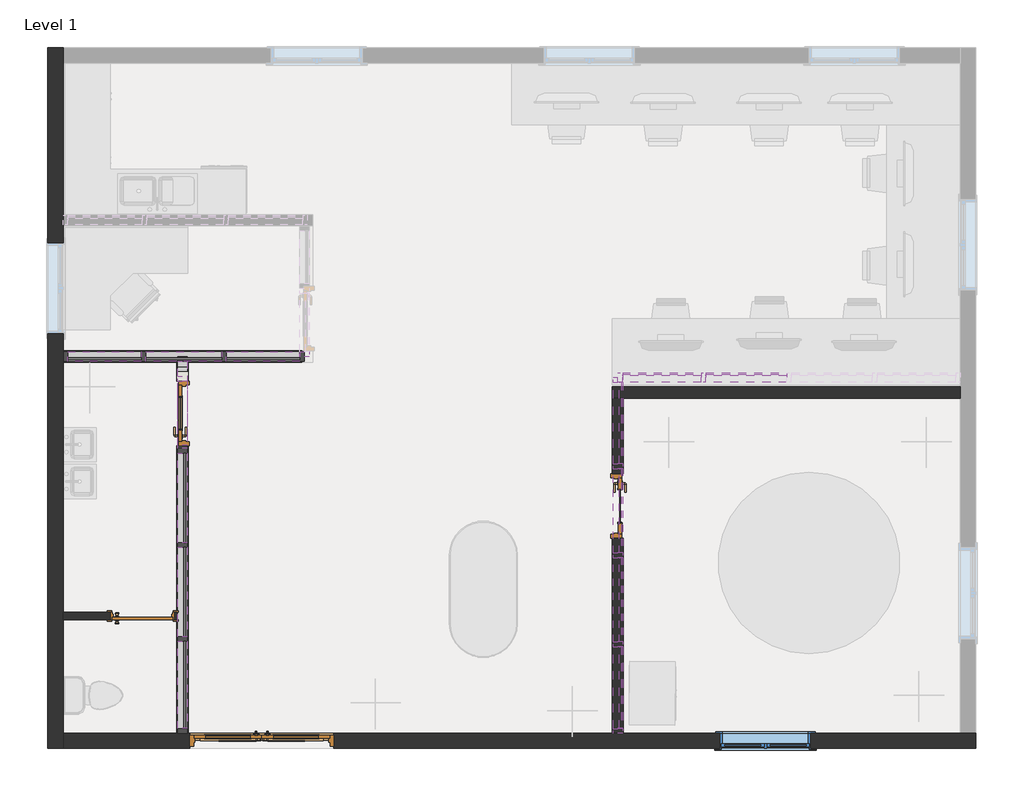
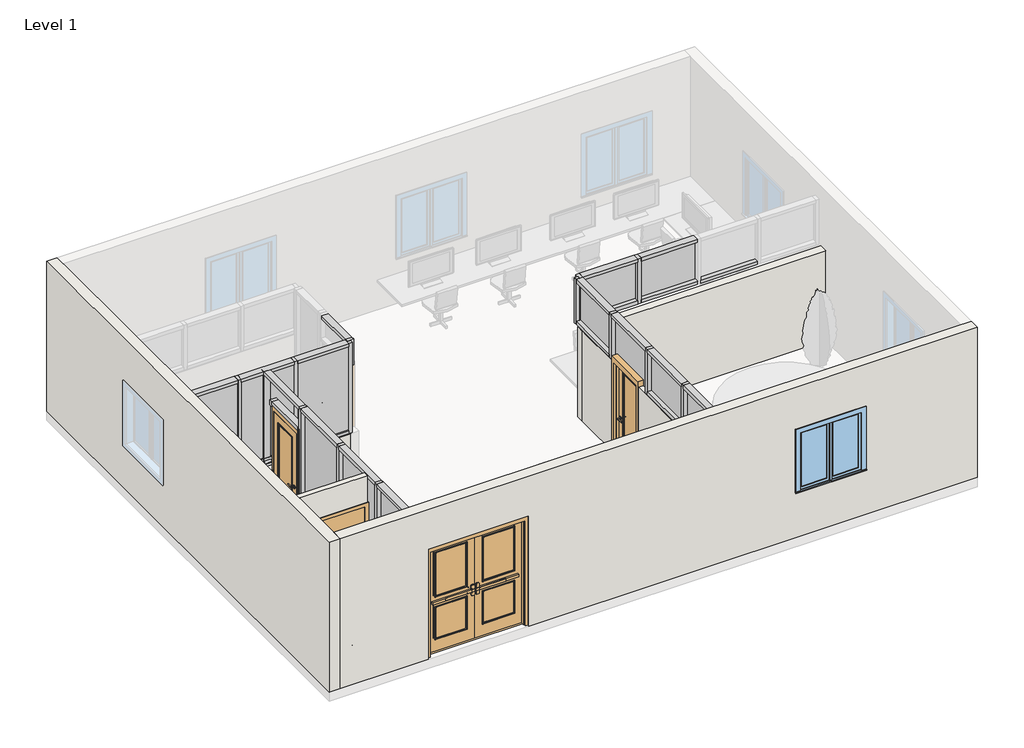
# One storey, part 1 of 2: 49 members, 12 plates, 7 walls, 4 doors, 1 window.
"""IFC4 building model written with IfcOpenShell, lengths in millimetres."""

from ifc_helpers import new_model, si_unit, frame, origin, origin_with_axes, place, context, project, spatial, polyline, outline, extrude, faceted_brep, transform, mapped, element, save
from components import door_6260e01d, door_549a8064, door_95a5efb1, door_3c591639, door_29f5c000, member_410c6227, member_73c23c35, member_7fa39cca, member_95280835, member_d60e8053, member_2fae0574, member_69c8e218, member_a08f6adc, member_3d7cb871, member_b70ee1cc, member_67d1cd44, member_476d3acb, member_e9c7f4a4, member_e1cf819f, member_429f6687, member_5446ee95, member_f5f6c3fe, member_8e09d03a, member_f1b77eba, system_panel_glazed_cfce8111, system_panel_glazed_768357cb, system_panel_glazed_3f576ca0, system_panel_glazed_47051e8e, system_panel_glazed_8590af86, system_panel_glazed_1700d241, system_panel_glazed_dd77c3d1, system_panel_glazed_5745033b, system_panel_glazed_e830b44b, window_0862ab64

model = new_model("IFC4")

# Units and contexts
model_context = context("Model", 3, world=origin())
ifc_project = project(units=[si_unit("LENGTHUNIT", "METRE", prefix="MILLI")], contexts=[model_context])

# Site, building, storey
site = spatial("IfcSite", under=ifc_project)
building = spatial("IfcBuilding", under=site)
storey = spatial("IfcBuildingStorey", under=building, Name="Level 1", Elevation=0.0)

# Doors
placement = place(None, origin())
door_shape = door_6260e01d(model_context)
door_2_shape = door_549a8064(model_context)
door_3_shape = door_95a5efb1(model_context)
element("IfcDoor", 1, ObjectType="Door-Exterior-Double-Two_Lite : 72\" x 84\"", at=placement, inside=storey, context=model_context, shape_type="MappedRepresentation", body=[
    mapped(door_shape, transform((7432.6010577, -13459.2708301, 0.0), x_axis=(1.0, 0.0, 0.0), y_axis=(0.0, 1.0, 0.0), z_axis=(0.0, 0.0, 1.0))),
    mapped(door_2_shape, transform((7432.6010577, -13459.2708301, 0.0), x_axis=(1.0, 0.0, 0.0), y_axis=(0.0, 1.0, 0.0), z_axis=(0.0, 0.0, 1.0))),
    mapped(door_3_shape, transform((7432.6010577, -13459.2708301, 0.0), x_axis=(1.0, 0.0, 0.0), y_axis=(0.0, 1.0, 0.0), z_axis=(0.0, 0.0, 1.0))),
])
door_4_shape = door_3c591639(model_context)
element("IfcDoor", 2, ObjectType="Door-Interior-Single-Flush_Panel-Wood : 32\" x 84\"", at=placement, inside=storey, context=model_context, shape_type="MappedRepresentation", body=[
    mapped(door_4_shape, transform((5832.4010577, -11779.6958301, 0.0), x_axis=(1.0, 0.0, 0.0), y_axis=(0.0, 1.0, 0.0), z_axis=(0.0, 0.0, 1.0))),
])
door_5_shape = door_29f5c000(model_context)
element("IfcDoor", 3, ObjectType="Door-Passage-Single-Full_Lite : 30\" x 84\"", at=placement, inside=storey, context=model_context, shape_type="MappedRepresentation", body=[
    mapped(door_5_shape, transform((12201.4510577, -10303.3208301, -284.48), x_axis=(0.0, -1.0, 0.0), y_axis=(1.0, 0.0, 0.0), z_axis=(0.0, 0.0, 1.0))),
])
element("IfcDoor", 4, ObjectType="Door-Passage-Single-Full_Lite : 30\" x 84\"", at=placement, inside=storey, context=model_context, shape_type="MappedRepresentation", body=[
    mapped(door_5_shape, transform((6372.1510577, -9058.7208301, 0.0), x_axis=(0.0, 1.0, 0.0), y_axis=(-1.0, 0.0, 0.0), z_axis=(0.0, 0.0, 1.0))),
])

# Members
member_shape = member_410c6227(model_context)
element("IfcMember", 5, ObjectType="Rectangular Mullion : 2.5\" x 5\" rectangular", at=placement, inside=storey, context=model_context, shape_type="MappedRepresentation", body=[
    mapped(member_shape, transform((13357.1510577, -8576.1208301, 1828.8), x_axis=(1.0, 0.0, 0.0), y_axis=(0.0, -1.0, 0.0), z_axis=(0.0, 0.0, -1.0))),
])
element("IfcMember", 6, ObjectType="Rectangular Mullion : 2.5\" x 5\" rectangular", at=placement, inside=storey, context=model_context, shape_type="MappedRepresentation", body=[
    mapped(member_shape, transform((12207.8010577, -9769.9208301, 1828.8), x_axis=(0.0, -1.0, 0.0), y_axis=(-1.0, 0.0, 0.0), z_axis=(0.0, 0.0, -1.0))),
])
element("IfcMember", 7, ObjectType="Rectangular Mullion : 2.5\" x 5\" rectangular", at=placement, inside=storey, context=model_context, shape_type="MappedRepresentation", body=[
    mapped(member_shape, transform((12207.8010577, -10963.7208301, 1828.8), x_axis=(0.0, -1.0, 0.0), y_axis=(-1.0, 0.0, 0.0), z_axis=(0.0, 0.0, -1.0))),
])
element("IfcMember", 8, ObjectType="Rectangular Mullion : 2.5\" x 5\" rectangular", at=placement, inside=storey, context=model_context, shape_type="MappedRepresentation", body=[
    mapped(member_shape, transform((12207.8010577, -12157.5208301, 1828.8), x_axis=(0.0, -1.0, 0.0), y_axis=(-1.0, 0.0, 0.0), z_axis=(0.0, 0.0, -1.0))),
])
member_2_shape = member_73c23c35(model_context)
element("IfcMember", 9, ObjectType="Rectangular Mullion : 2.5\" x 5\" rectangular", at=placement, inside=storey, context=model_context, shape_type="MappedRepresentation", body=[
    mapped(member_2_shape, transform((12207.8010577, -13351.3208301, 1828.8), x_axis=(0.0, -1.0, 0.0), y_axis=(-1.0, 0.0, 0.0), z_axis=(0.0, 0.0, -1.0))),
])
element("IfcMember", 10, ObjectType="Rectangular Mullion : 2.5\" x 5\" rectangular", at=placement, inside=storey, context=model_context, shape_type="MappedRepresentation", body=[
    mapped(member_2_shape, transform((12207.8010577, -8576.1208301, 2743.2), x_axis=(-1.0, 0.0, 0.0), y_axis=(0.0, -1.0, 0.0), z_axis=(0.0, 0.0, 1.0))),
])
element("IfcMember", 11, ObjectType="Rectangular Mullion : 2.5\" x 5\" rectangular", at=placement, inside=storey, context=model_context, shape_type="MappedRepresentation", body=[
    mapped(member_2_shape, transform((12207.8010577, -8576.1208301, 2743.2), x_axis=(0.0, 1.0, 0.0), y_axis=(-1.0, 0.0, 0.0), z_axis=(0.0, 0.0, 1.0))),
])
member_3_shape = member_7fa39cca(model_context)
element("IfcMember", 12, ObjectType="Rectangular Mullion : 2.5\" x 5\" rectangular", at=placement, inside=storey, context=model_context, shape_type="MappedRepresentation", body=[
    mapped(member_3_shape, transform((13325.4010577, -8576.1208301, 2743.2), x_axis=(0.0, 0.0, 1.0), y_axis=(0.0, -1.0, 0.0), z_axis=(1.0, 0.0, 0.0))),
])
member_4_shape = member_95280835(model_context)
element("IfcMember", 13, ObjectType="Rectangular Mullion : 2.5\" x 5\" rectangular", at=placement, inside=storey, context=model_context, shape_type="MappedRepresentation", body=[
    mapped(member_4_shape, transform((14474.7510577, -8576.1208301, 2743.2), x_axis=(0.0, 0.0, 1.0), y_axis=(0.0, -1.0, 0.0), z_axis=(1.0, 0.0, 0.0))),
])
element("IfcMember", 14, ObjectType="Rectangular Mullion : 2.5\" x 5\" rectangular", at=placement, inside=storey, context=model_context, shape_type="MappedRepresentation", body=[
    mapped(member_3_shape, transform((12271.3010577, -8576.1208301, 1828.8), x_axis=(0.0, 0.0, -1.0), y_axis=(0.0, -1.0, 0.0), z_axis=(-1.0, 0.0, 0.0))),
])
element("IfcMember", 15, ObjectType="Rectangular Mullion : 2.5\" x 5\" rectangular", at=placement, inside=storey, context=model_context, shape_type="MappedRepresentation", body=[
    mapped(member_4_shape, transform((13388.9010577, -8576.1208301, 1828.8), x_axis=(0.0, 0.0, -1.0), y_axis=(0.0, -1.0, 0.0), z_axis=(-1.0, 0.0, 0.0))),
])
element("IfcMember", 16, ObjectType="Rectangular Mullion : 2.5\" x 5\" rectangular", at=placement, inside=storey, context=model_context, shape_type="MappedRepresentation", body=[
    mapped(member_4_shape, transform((14538.2510577, -8576.1208301, 1828.8), x_axis=(0.0, 0.0, -1.0), y_axis=(0.0, -1.0, 0.0), z_axis=(-1.0, 0.0, 0.0))),
])
member_5_shape = member_d60e8053(model_context)
element("IfcMember", 17, ObjectType="Rectangular Mullion : 2.5\" x 5\" rectangular", at=placement, inside=storey, context=model_context, shape_type="MappedRepresentation", body=[
    mapped(member_5_shape, transform((6924.6010577, -8296.7208301, 914.4), x_axis=(-1.0, 0.0, 0.0), y_axis=(0.0, 1.0, 0.0), z_axis=(0.0, 0.0, -1.0))),
])
element("IfcMember", 18, ObjectType="Rectangular Mullion : 2.5\" x 5\" rectangular", at=placement, inside=storey, context=model_context, shape_type="MappedRepresentation", body=[
    mapped(member_5_shape, transform((5845.1010577, -8296.7208301, 914.4), x_axis=(-1.0, 0.0, 0.0), y_axis=(0.0, 1.0, 0.0), z_axis=(0.0, 0.0, -1.0))),
])
element("IfcMember", 19, ObjectType="Rectangular Mullion : 2.5\" x 5\" rectangular", at=placement, inside=storey, context=model_context, shape_type="MappedRepresentation", body=[
    mapped(member_5_shape, transform((6365.8010577, -9560.3708301, 914.4), x_axis=(0.0, -1.0, 0.0), y_axis=(-1.0, 0.0, 0.0), z_axis=(0.0, 0.0, -1.0))),
])
element("IfcMember", 20, ObjectType="Rectangular Mullion : 2.5\" x 5\" rectangular", at=placement, inside=storey, context=model_context, shape_type="MappedRepresentation", body=[
    mapped(member_5_shape, transform((6365.8010577, -10824.0208301, 914.4), x_axis=(0.0, -1.0, 0.0), y_axis=(-1.0, 0.0, 0.0), z_axis=(0.0, 0.0, -1.0))),
])
element("IfcMember", 21, ObjectType="Rectangular Mullion : 2.5\" x 5\" rectangular", at=placement, inside=storey, context=model_context, shape_type="MappedRepresentation", body=[
    mapped(member_5_shape, transform((6365.8010577, -12087.6708301, 914.4), x_axis=(0.0, -1.0, 0.0), y_axis=(-1.0, 0.0, 0.0), z_axis=(0.0, 0.0, -1.0))),
])
member_6_shape = member_2fae0574(model_context)
element("IfcMember", 22, ObjectType="Rectangular Mullion : 2.5\" x 5\" rectangular", at=placement, inside=storey, context=model_context, shape_type="MappedRepresentation", body=[
    mapped(member_6_shape, transform((4765.6010577, -8296.7208301, 914.4), x_axis=(-1.0, 0.0, 0.0), y_axis=(0.0, 1.0, 0.0), z_axis=(0.0, 0.0, -1.0))),
])
element("IfcMember", 23, ObjectType="Rectangular Mullion : 2.5\" x 5\" rectangular", at=placement, inside=storey, context=model_context, shape_type="MappedRepresentation", body=[
    mapped(member_6_shape, transform((6365.8010577, -13351.3208301, 914.4), x_axis=(0.0, -1.0, 0.0), y_axis=(-1.0, 0.0, 0.0), z_axis=(0.0, 0.0, -1.0))),
])
element("IfcMember", 24, ObjectType="Rectangular Mullion : 2.5\" x 5\" rectangular", at=placement, inside=storey, context=model_context, shape_type="MappedRepresentation", body=[
    mapped(member_6_shape, transform((8004.1010577, -8296.7208301, 2743.2), x_axis=(1.0, 0.0, 0.0), y_axis=(0.0, 1.0, 0.0), z_axis=(0.0, 0.0, 1.0))),
])
member_7_shape = member_69c8e218(model_context)
element("IfcMember", 25, ObjectType="Rectangular Mullion : 2.5\" x 5\" rectangular", at=placement, inside=storey, context=model_context, shape_type="MappedRepresentation", body=[
    mapped(member_7_shape, transform((12207.8010577, -13287.8208301, 2743.2), x_axis=(0.0, 0.0, 1.0), y_axis=(-1.0, 0.0, 0.0), z_axis=(0.0, -1.0, 0.0))),
])
element("IfcMember", 26, ObjectType="Rectangular Mullion : 2.5\" x 5\" rectangular", at=placement, inside=storey, context=model_context, shape_type="MappedRepresentation", body=[
    mapped(member_7_shape, transform((12207.8010577, -9738.1708301, 2743.2), x_axis=(0.0, 0.0, 1.0), y_axis=(-1.0, 0.0, 0.0), z_axis=(0.0, -1.0, 0.0))),
])
member_8_shape = member_a08f6adc(model_context)
element("IfcMember", 27, ObjectType="Rectangular Mullion : 2.5\" x 5\" rectangular", at=placement, inside=storey, context=model_context, shape_type="MappedRepresentation", body=[
    mapped(member_8_shape, transform((12207.8010577, -10931.9708301, 2743.2), x_axis=(0.0, 0.0, 1.0), y_axis=(-1.0, 0.0, 0.0), z_axis=(0.0, -1.0, 0.0))),
])
element("IfcMember", 28, ObjectType="Rectangular Mullion : 2.5\" x 5\" rectangular", at=placement, inside=storey, context=model_context, shape_type="MappedRepresentation", body=[
    mapped(member_8_shape, transform((12207.8010577, -12125.7708301, 2743.2), x_axis=(0.0, 0.0, 1.0), y_axis=(-1.0, 0.0, 0.0), z_axis=(0.0, -1.0, 0.0))),
])
element("IfcMember", 29, ObjectType="Rectangular Mullion : 2.5\" x 5\" rectangular", at=placement, inside=storey, context=model_context, shape_type="MappedRepresentation", body=[
    mapped(member_7_shape, transform((12207.8010577, -8639.6208301, 1828.8), x_axis=(0.0, 0.0, -1.0), y_axis=(-1.0, 0.0, 0.0), z_axis=(0.0, 1.0, 0.0))),
])
element("IfcMember", 30, ObjectType="Rectangular Mullion : 2.5\" x 5\" rectangular", at=placement, inside=storey, context=model_context, shape_type="MappedRepresentation", body=[
    mapped(member_7_shape, transform((12207.8010577, -12189.2708301, 1828.8), x_axis=(0.0, 0.0, -1.0), y_axis=(-1.0, 0.0, 0.0), z_axis=(0.0, 1.0, 0.0))),
])
element("IfcMember", 31, ObjectType="Rectangular Mullion : 2.5\" x 5\" rectangular", at=placement, inside=storey, context=model_context, shape_type="MappedRepresentation", body=[
    mapped(member_8_shape, transform((12207.8010577, -10995.4708301, 1828.8), x_axis=(0.0, 0.0, -1.0), y_axis=(-1.0, 0.0, 0.0), z_axis=(0.0, 1.0, 0.0))),
])
member_9_shape = member_3d7cb871(model_context)
element("IfcMember", 32, ObjectType="Rectangular Mullion : 2.5\" x 5\" rectangular", at=placement, inside=storey, context=model_context, shape_type="MappedRepresentation", body=[
    mapped(member_9_shape, transform((6365.8010577, -8360.2208301, 863.6), x_axis=(0.0, 0.0, -1.0), y_axis=(-1.0, 0.0, 0.0), z_axis=(0.0, 1.0, 0.0))),
])
member_10_shape = member_b70ee1cc(model_context)
element("IfcMember", 33, ObjectType="Rectangular Mullion : 2.5\" x 5\" rectangular", at=placement, inside=storey, context=model_context, shape_type="MappedRepresentation", body=[
    mapped(member_10_shape, transform((6365.8010577, -8626.9208301, 2235.2), x_axis=(0.0, 0.0, -1.0), y_axis=(-1.0, 0.0, 0.0), z_axis=(0.0, 1.0, 0.0))),
])
element("IfcMember", 34, ObjectType="Rectangular Mullion : 2.5\" x 5\" rectangular", at=placement, inside=storey, context=model_context, shape_type="MappedRepresentation", body=[
    mapped(member_6_shape, transform((6365.8010577, -8296.7208301, 2743.2), x_axis=(0.0, 1.0, 0.0), y_axis=(-1.0, 0.0, 0.0), z_axis=(0.0, 0.0, 1.0))),
])
member_11_shape = member_67d1cd44(model_context)
element("IfcMember", 35, ObjectType="Rectangular Mullion : 2.5\" x 5\" rectangular", at=placement, inside=storey, context=model_context, shape_type="MappedRepresentation", body=[
    mapped(member_11_shape, transform((6365.8010577, -8296.7208301, 914.4), x_axis=(0.0, 1.0, 0.0), y_axis=(-1.0, 0.0, 0.0), z_axis=(0.0, 0.0, 1.0))),
])
member_12_shape = member_476d3acb(model_context)
element("IfcMember", 36, ObjectType="Rectangular Mullion : 2.5\" x 5\" rectangular", at=placement, inside=storey, context=model_context, shape_type="MappedRepresentation", body=[
    mapped(member_12_shape, transform((6365.8010577, -13287.8208301, 2743.2), x_axis=(0.0, 0.0, 1.0), y_axis=(-1.0, 0.0, 0.0), z_axis=(0.0, -1.0, 0.0))),
])
element("IfcMember", 37, ObjectType="Rectangular Mullion : 2.5\" x 5\" rectangular", at=placement, inside=storey, context=model_context, shape_type="MappedRepresentation", body=[
    mapped(member_12_shape, transform((6365.8010577, -9528.6208301, 2743.2), x_axis=(0.0, 0.0, 1.0), y_axis=(-1.0, 0.0, 0.0), z_axis=(0.0, -1.0, 0.0))),
])
member_13_shape = member_e9c7f4a4(model_context)
element("IfcMember", 38, ObjectType="Rectangular Mullion : 2.5\" x 5\" rectangular", at=placement, inside=storey, context=model_context, shape_type="MappedRepresentation", body=[
    mapped(member_13_shape, transform((6365.8010577, -10792.2708301, 2743.2), x_axis=(0.0, 0.0, 1.0), y_axis=(-1.0, 0.0, 0.0), z_axis=(0.0, -1.0, 0.0))),
])
element("IfcMember", 39, ObjectType="Rectangular Mullion : 2.5\" x 5\" rectangular", at=placement, inside=storey, context=model_context, shape_type="MappedRepresentation", body=[
    mapped(member_13_shape, transform((6365.8010577, -12055.9208301, 2743.2), x_axis=(0.0, 0.0, 1.0), y_axis=(-1.0, 0.0, 0.0), z_axis=(0.0, -1.0, 0.0))),
])
element("IfcMember", 40, ObjectType="Rectangular Mullion : 2.5\" x 5\" rectangular", at=placement, inside=storey, context=model_context, shape_type="MappedRepresentation", body=[
    mapped(member_13_shape, transform((6365.8010577, -9592.1208301, 914.4), x_axis=(0.0, 0.0, -1.0), y_axis=(-1.0, 0.0, 0.0), z_axis=(0.0, 1.0, 0.0))),
])
element("IfcMember", 41, ObjectType="Rectangular Mullion : 2.5\" x 5\" rectangular", at=placement, inside=storey, context=model_context, shape_type="MappedRepresentation", body=[
    mapped(member_13_shape, transform((6365.8010577, -10855.7708301, 914.4), x_axis=(0.0, 0.0, -1.0), y_axis=(-1.0, 0.0, 0.0), z_axis=(0.0, 1.0, 0.0))),
])
element("IfcMember", 42, ObjectType="Rectangular Mullion : 2.5\" x 5\" rectangular", at=placement, inside=storey, context=model_context, shape_type="MappedRepresentation", body=[
    mapped(member_12_shape, transform((6365.8010577, -12119.4208301, 914.4), x_axis=(0.0, 0.0, -1.0), y_axis=(-1.0, 0.0, 0.0), z_axis=(0.0, 1.0, 0.0))),
])
member_14_shape = member_e1cf819f(model_context)
element("IfcMember", 43, ObjectType="Rectangular Mullion : 2.5\" x 5\" rectangular", at=placement, inside=storey, context=model_context, shape_type="MappedRepresentation", body=[
    mapped(member_14_shape, transform((6365.8010577, -9490.5208301, 2298.7), x_axis=(0.0, 1.0, 0.0), y_axis=(-1.0, 0.0, 0.0), z_axis=(0.0, 0.0, 1.0))),
])
member_15_shape = member_429f6687(model_context)
element("IfcMember", 44, ObjectType="Rectangular Mullion : 2.5\" x 5\" rectangular", at=placement, inside=storey, context=model_context, shape_type="MappedRepresentation", body=[
    mapped(member_15_shape, transform((8004.1010577, -8233.2208301, 2754.1090709), x_axis=(0.0, 0.0, 1.0), y_axis=(-1.0, 0.0, 0.0), z_axis=(0.0, -1.0, 0.0))),
])
element("IfcMember", 45, ObjectType="Rectangular Mullion : 2.5\" x 5\" rectangular", at=placement, inside=storey, context=model_context, shape_type="MappedRepresentation", body=[
    mapped(member_11_shape, transform((6365.8010577, -8499.9208301, 863.6), x_axis=(0.0, -1.0, 0.0), y_axis=(-1.0, 0.0, 0.0), z_axis=(0.0, 0.0, -1.0))),
])
member_16_shape = member_5446ee95(model_context)
element("IfcMember", 46, ObjectType="Rectangular Mullion : 2.5\" x 5\" rectangular", at=placement, inside=storey, context=model_context, shape_type="MappedRepresentation", body=[
    mapped(member_16_shape, transform((6365.8010577, -8626.9208301, 2197.7952723), x_axis=(0.0, -1.0, 0.0), y_axis=(-1.0, 0.0, 0.0), z_axis=(0.0, 0.0, -1.0))),
])
member_17_shape = member_f5f6c3fe(model_context)
element("IfcMember", 47, ObjectType="Rectangular Mullion : 2.5\" x 5\" rectangular", at=placement, inside=storey, context=model_context, shape_type="MappedRepresentation", body=[
    mapped(member_17_shape, transform((4829.1010577, -8296.7208301, 2743.2), x_axis=(0.0, 0.0, 1.0), y_axis=(0.0, 1.0, 0.0), z_axis=(-1.0, 0.0, 0.0))),
])
element("IfcMember", 48, ObjectType="Rectangular Mullion : 2.5\" x 5\" rectangular", at=placement, inside=storey, context=model_context, shape_type="MappedRepresentation", body=[
    mapped(member_17_shape, transform((6956.3510577, -8296.7208301, 2743.2), x_axis=(0.0, 0.0, 1.0), y_axis=(0.0, 1.0, 0.0), z_axis=(-1.0, 0.0, 0.0))),
])
member_18_shape = member_8e09d03a(model_context)
element("IfcMember", 49, ObjectType="Rectangular Mullion : 2.5\" x 5\" rectangular", at=placement, inside=storey, context=model_context, shape_type="MappedRepresentation", body=[
    mapped(member_18_shape, transform((5876.8510577, -8296.7208301, 2743.2), x_axis=(0.0, 0.0, 1.0), y_axis=(0.0, 1.0, 0.0), z_axis=(-1.0, 0.0, 0.0))),
])
element("IfcMember", 50, ObjectType="Rectangular Mullion : 2.5\" x 5\" rectangular", at=placement, inside=storey, context=model_context, shape_type="MappedRepresentation", body=[
    mapped(member_17_shape, transform((7940.6010577, -8296.7208301, 914.4), x_axis=(0.0, 0.0, -1.0), y_axis=(0.0, 1.0, 0.0), z_axis=(1.0, 0.0, 0.0))),
])
element("IfcMember", 51, ObjectType="Rectangular Mullion : 2.5\" x 5\" rectangular", at=placement, inside=storey, context=model_context, shape_type="MappedRepresentation", body=[
    mapped(member_17_shape, transform((5813.3510577, -8296.7208301, 914.4), x_axis=(0.0, 0.0, -1.0), y_axis=(0.0, 1.0, 0.0), z_axis=(1.0, 0.0, 0.0))),
])
element("IfcMember", 52, ObjectType="Rectangular Mullion : 2.5\" x 5\" rectangular", at=placement, inside=storey, context=model_context, shape_type="MappedRepresentation", body=[
    mapped(member_18_shape, transform((6892.8510577, -8296.7208301, 914.4), x_axis=(0.0, 0.0, -1.0), y_axis=(0.0, 1.0, 0.0), z_axis=(1.0, 0.0, 0.0))),
])
member_19_shape = member_f1b77eba(model_context)
element("IfcMember", 53, ObjectType="Rectangular Mullion : 2.5\" x 5\" rectangular", at=placement, inside=storey, context=model_context, shape_type="MappedRepresentation", body=[
    mapped(member_19_shape, transform((8004.1010577, -8296.7208301, 2235.2), x_axis=(0.0, -1.0, 0.0), y_axis=(-1.0, 0.0, 0.0), z_axis=(0.0, 0.0, -1.0))),
])

# Plates
system_panel_glazed_shape = system_panel_glazed_cfce8111(model_context)
element("IfcPlate", 54, ObjectType="System Panel : Glazed", at=placement, inside=storey, context=model_context, shape_type="MappedRepresentation", body=[
    mapped(system_panel_glazed_shape, transform((12798.3510577, -8576.1208301, 1892.3), x_axis=(1.0, 0.0, 0.0), y_axis=(0.0, 1.0, 0.0), z_axis=(0.0, 0.0, 1.0))),
])
system_panel_glazed_2_shape = system_panel_glazed_768357cb(model_context)
element("IfcPlate", 55, ObjectType="System Panel : Glazed", at=placement, inside=storey, context=model_context, shape_type="MappedRepresentation", body=[
    mapped(system_panel_glazed_2_shape, transform((13931.8260577, -8576.1208301, 1892.3), x_axis=(1.0, 0.0, 0.0), y_axis=(0.0, 1.0, 0.0), z_axis=(0.0, 0.0, 1.0))),
])
system_panel_glazed_3_shape = system_panel_glazed_3f576ca0(model_context)
element("IfcPlate", 56, ObjectType="System Panel : Glazed", at=placement, inside=storey, context=model_context, shape_type="MappedRepresentation", body=[
    mapped(system_panel_glazed_3_shape, transform((12207.8010577, -9188.8958301, 1892.3), x_axis=(0.0, -1.0, 0.0), y_axis=(1.0, 0.0, 0.0), z_axis=(0.0, 0.0, 1.0))),
])
element("IfcPlate", 57, ObjectType="System Panel : Glazed", at=placement, inside=storey, context=model_context, shape_type="MappedRepresentation", body=[
    mapped(system_panel_glazed_3_shape, transform((12207.8010577, -12738.5458301, 1892.3), x_axis=(0.0, -1.0, 0.0), y_axis=(1.0, 0.0, 0.0), z_axis=(0.0, 0.0, 1.0))),
])
system_panel_glazed_4_shape = system_panel_glazed_47051e8e(model_context)
element("IfcPlate", 58, ObjectType="System Panel : Glazed", at=placement, inside=storey, context=model_context, shape_type="MappedRepresentation", body=[
    mapped(system_panel_glazed_4_shape, transform((12207.8010577, -11560.6208301, 1892.3), x_axis=(0.0, -1.0, 0.0), y_axis=(1.0, 0.0, 0.0), z_axis=(0.0, 0.0, 1.0))),
])
system_panel_glazed_5_shape = system_panel_glazed_8590af86(model_context)
element("IfcPlate", 59, ObjectType="System Panel : Glazed", at=placement, inside=storey, context=model_context, shape_type="MappedRepresentation", body=[
    mapped(system_panel_glazed_5_shape, transform((6365.8010577, -10192.1958301, 977.9), x_axis=(0.0, -1.0, 0.0), y_axis=(1.0, 0.0, 0.0), z_axis=(0.0, 0.0, 1.0))),
])
element("IfcPlate", 60, ObjectType="System Panel : Glazed", at=placement, inside=storey, context=model_context, shape_type="MappedRepresentation", body=[
    mapped(system_panel_glazed_5_shape, transform((6365.8010577, -11455.8458301, 977.9), x_axis=(0.0, -1.0, 0.0), y_axis=(1.0, 0.0, 0.0), z_axis=(0.0, 0.0, 1.0))),
])
system_panel_glazed_6_shape = system_panel_glazed_1700d241(model_context)
element("IfcPlate", 61, ObjectType="System Panel : Glazed", at=placement, inside=storey, context=model_context, shape_type="MappedRepresentation", body=[
    mapped(system_panel_glazed_6_shape, transform((6365.8010577, -12703.6208301, 977.9), x_axis=(0.0, -1.0, 0.0), y_axis=(1.0, 0.0, 0.0), z_axis=(0.0, 0.0, 1.0))),
])
system_panel_glazed_7_shape = system_panel_glazed_dd77c3d1(model_context)
element("IfcPlate", 62, ObjectType="System Panel : Glazed", at=placement, inside=storey, context=model_context, shape_type="MappedRepresentation", body=[
    mapped(system_panel_glazed_7_shape, transform((12207.8010577, -10366.8208301, 1828.8), x_axis=(0.0, -1.0, 0.0), y_axis=(1.0, 0.0, 0.0), z_axis=(0.0, 0.0, 1.0))),
])
system_panel_glazed_8_shape = system_panel_glazed_5745033b(model_context)
element("IfcPlate", 63, ObjectType="System Panel : Glazed", at=placement, inside=storey, context=model_context, shape_type="MappedRepresentation", body=[
    mapped(system_panel_glazed_8_shape, transform((7448.4760577, -8296.7208301, 977.9), x_axis=(-1.0, 0.0, 0.0), y_axis=(0.0, -1.0, 0.0), z_axis=(0.0, 0.0, 1.0))),
])
element("IfcPlate", 64, ObjectType="System Panel : Glazed", at=placement, inside=storey, context=model_context, shape_type="MappedRepresentation", body=[
    mapped(system_panel_glazed_8_shape, transform((5321.2260577, -8296.7208301, 977.9), x_axis=(-1.0, 0.0, 0.0), y_axis=(0.0, -1.0, 0.0), z_axis=(0.0, 0.0, 1.0))),
])
system_panel_glazed_9_shape = system_panel_glazed_e830b44b(model_context)
element("IfcPlate", 65, ObjectType="System Panel : Glazed", at=placement, inside=storey, context=model_context, shape_type="MappedRepresentation", body=[
    mapped(system_panel_glazed_9_shape, transform((6384.8510577, -8296.7208301, 977.9), x_axis=(-1.0, 0.0, 0.0), y_axis=(0.0, -1.0, 0.0), z_axis=(0.0, 0.0, 1.0))),
])

# Walls
element("IfcWall", 66, ObjectType="Generic - 4\" Brick", at=placement, inside=storey, context=model_context, shape_type="SweptSolid", body=[
    extrude(outline(polyline([(2743.2, 6289.6010577), (2743.2, 4765.6010577), (0.0, 4765.6010577), (0.0, 5400.6010577), (2159.0, 5400.6010577), (2159.0, 6264.2010577), (0.0, 6264.2010577), (0.0, 6289.6010577), (2743.2, 6289.6010577)])), frame((0.0, -11827.3208301, 0.0), z_axis=(0.0, 1.0, 0.0), x_axis=(0.0, 0.0, 1.0)), (0.0, 0.0, 1.0), 101.6),
])
element("IfcWall", 67, ObjectType="Generic - 6\"", at=placement, inside=storey, context=model_context, shape_type="Brep", body=[
    faceted_brep([(7966.0010577, -8220.5208301, 0.0), (4765.6010577, -8220.5208301, 0.0), (4765.6010577, -8220.5208301, 914.4), (7966.0010577, -8220.5208301, 914.4), (7966.0010577, -8372.9208301, 0.0), (7966.0010577, -8372.9208301, 914.4), (6442.0010577, -8372.9208301, 914.4), (6289.6010577, -8372.9208301, 914.4), (4765.6010577, -8372.9208301, 914.4), (4765.6010577, -8372.9208301, 0.0), (6289.6010577, -8372.9208301, 0.0), (6442.0010577, -8372.9208301, 0.0)], [[[0, 1, 2, 3]], [[4, 5, 6, 7, 8, 9, 10, 11]], [[1, 0, 4, 11, 10, 9]], [[3, 2, 8, 7, 6, 5]], [[0, 3, 5, 4]], [[2, 1, 9, 8]]]),
])
element("IfcWall", 68, ObjectType="Generic - 6\"", at=placement, inside=storey, context=model_context, shape_type="Brep", body=[
    faceted_brep([(6289.6010577, -13351.3208301, 0.0), (6289.6010577, -13351.3208301, 914.4), (6289.6010577, -9490.5208301, 914.4), (6289.6010577, -9490.5208301, 0.0), (6289.6010577, -11725.7208301, 0.0), (6289.6010577, -11827.3208301, 0.0), (6442.0010577, -13351.3208301, 914.4), (6442.0010577, -13351.3208301, 0.0), (6442.0010577, -9490.5208301, 0.0), (6442.0010577, -9490.5208301, 914.4)], [[[0, 1, 2, 3, 4, 5]], [[6, 7, 8, 9]], [[7, 0, 5, 4, 3, 8]], [[1, 6, 9, 2]], [[1, 0, 7, 6]], [[3, 2, 9, 8]]]),
    faceted_brep([(6289.6010577, -8372.9208301, 0.0), (6289.6010577, -8626.9208301, 0.0), (6289.6010577, -8626.9208301, 914.4), (6289.6010577, -8499.9208301, 914.4), (6289.6010577, -8499.9208301, 863.6), (6289.6010577, -8372.9208301, 863.6), (6442.0010577, -8626.9208301, 0.0), (6442.0010577, -8372.9208301, 0.0), (6442.0010577, -8372.9208301, 863.6), (6442.0010577, -8499.9208301, 863.6), (6442.0010577, -8499.9208301, 914.4), (6442.0010577, -8626.9208301, 914.4)], [[[0, 1, 2, 3, 4, 5]], [[6, 7, 8, 9, 10, 11]], [[0, 7, 6, 1]], [[2, 11, 10, 3]], [[7, 0, 5, 8]], [[2, 1, 6, 11]], [[9, 4, 3, 10]], [[4, 9, 8, 5]]]),
])
element("IfcWall", 69, ObjectType="Generic - 6\"", at=placement, inside=storey, context=model_context, shape_type="Brep", body=[
    faceted_brep([(16805.2010577, -8703.1208301, 0.0), (12131.6010577, -8703.1208301, 0.0), (12131.6010577, -8703.1208301, 1828.8), (16805.2010577, -8703.1208301, 1828.8), (16805.2010577, -8855.5208301, 0.0), (16805.2010577, -8855.5208301, 1828.8), (12284.0010577, -8855.5208301, 1828.8), (12131.6010577, -8855.5208301, 1828.8), (12131.6010577, -8855.5208301, 0.0), (12284.0010577, -8855.5208301, 0.0)], [[[0, 1, 2, 3]], [[4, 5, 6, 7, 8, 9]], [[1, 0, 4, 9, 8]], [[3, 2, 7, 6, 5]], [[0, 3, 5, 4]], [[2, 1, 8, 7]]]),
])
element("IfcWall", 70, ObjectType="Generic - 6\"", at=placement, inside=storey, context=model_context, shape_type="SweptSolid", body=[
    extrude(outline(polyline([(12284.0010577, -13351.3208301), (12131.6010577, -13351.3208301), (12131.6010577, -10735.1208301), (12284.0010577, -10735.1208301), (12284.0010577, -13351.3208301)])), origin_with_axes(), (0.0, 0.0, 1.0), 1828.8),
    extrude(outline(polyline([(12131.6010577, -8855.5208301), (12284.0010577, -8855.5208301), (12284.0010577, -9871.5208301), (12131.6010577, -9871.5208301), (12131.6010577, -8855.5208301)])), origin_with_axes(), (0.0, 0.0, 1.0), 1828.8),
])
element("IfcWall", 71, ObjectType="Generic - 8\"", at=placement, inside=storey, context=model_context, shape_type="Brep", body=[
    faceted_brep([(4562.4010577, -4156.5208301, 0.0), (4562.4010577, -13554.5208301, 0.0), (4562.4010577, -13554.5208301, 3048.0), (4562.4010577, -4156.5208301, 3048.0), (4562.4010577, -7991.9208301, 2133.6), (4562.4010577, -7991.9208301, 914.4), (4562.4010577, -6772.7208301, 914.4), (4562.4010577, -6772.7208301, 2133.6), (4765.6010577, -4156.5208301, 0.0), (4765.6010577, -4156.5208301, 3048.0), (4765.6010577, -4359.7208301, 3048.0), (4765.6010577, -13351.3208301, 3048.0), (4765.6010577, -13554.5208301, 3048.0), (4765.6010577, -13554.5208301, 0.0), (4765.6010577, -13351.3208301, 0.0), (4765.6010577, -11827.3208301, 0.0), (4765.6010577, -11725.7208301, 0.0), (4765.6010577, -8372.9208301, 0.0), (4765.6010577, -8220.5208301, 0.0), (4765.6010577, -6544.1208301, 0.0), (4765.6010577, -6391.7208301, 0.0), (4765.6010577, -4359.7208301, 0.0), (4765.6010577, -7991.9208301, 2133.6), (4765.6010577, -6772.7208301, 2133.6), (4765.6010577, -6772.7208301, 914.4), (4765.6010577, -7991.9208301, 914.4)], [[[0, 1, 2, 3], [4, 5, 6, 7]], [[8, 9, 10, 11, 12, 13, 14, 15, 16, 17, 18, 19, 20, 21], [22, 23, 24, 25]], [[1, 0, 8, 21, 20, 19, 18, 17, 16, 15, 14, 13]], [[3, 2, 12, 11, 10, 9]], [[2, 1, 13, 12]], [[0, 3, 9, 8]], [[5, 4, 22, 25]], [[6, 5, 25, 24]], [[7, 6, 24, 23]], [[4, 7, 23, 22]]]),
])
element("IfcWall", 72, ObjectType="Generic - 8\"", at=placement, inside=storey, context=model_context, shape_type="Brep", body=[
    faceted_brep([(17008.4010577, -13554.5208301, 3048.0), (4765.6010577, -13554.5208301, 3048.0), (4765.6010577, -13554.5208301, 0.0), (6467.4010577, -13554.5208301, 0.0), (6467.4010577, -13554.5208301, 2235.2), (8397.8010577, -13554.5208301, 2235.2), (8397.8010577, -13554.5208301, 0.0), (17008.4010577, -13554.5208301, 0.0), (13579.4010577, -13554.5208301, 2133.6), (14798.6010577, -13554.5208301, 2133.6), (14798.6010577, -13554.5208301, 914.4), (13579.4010577, -13554.5208301, 914.4), (4765.6010577, -13351.3208301, 3048.0), (16805.2010577, -13351.3208301, 3048.0), (17008.4010577, -13351.3208301, 3048.0), (17008.4010577, -13351.3208301, 0.0), (16805.2010577, -13351.3208301, 0.0), (12284.0010577, -13351.3208301, 0.0), (12131.6010577, -13351.3208301, 0.0), (8397.8010577, -13351.3208301, 0.0), (8397.8010577, -13351.3208301, 2235.2), (6467.4010577, -13351.3208301, 2235.2), (6467.4010577, -13351.3208301, 0.0), (6442.0010577, -13351.3208301, 0.0), (6289.6010577, -13351.3208301, 0.0), (4765.6010577, -13351.3208301, 0.0), (13579.4010577, -13351.3208301, 2133.6), (13579.4010577, -13351.3208301, 914.4), (14798.6010577, -13351.3208301, 914.4), (14798.6010577, -13351.3208301, 2133.6)], [[[0, 1, 2, 3, 4, 5, 6, 7], [8, 9, 10, 11]], [[12, 13, 14, 15, 16, 17, 18, 19, 20, 21, 22, 23, 24, 25], [26, 27, 28, 29]], [[2, 25, 24, 23, 22, 3]], [[15, 7, 6, 19, 18, 17, 16]], [[1, 0, 14, 13, 12]], [[2, 1, 12, 25]], [[0, 7, 15, 14]], [[5, 20, 19, 6]], [[20, 5, 4, 21]], [[21, 4, 3, 22]], [[27, 26, 8, 11]], [[28, 27, 11, 10]], [[29, 28, 10, 9]], [[26, 29, 9, 8]]]),
])

# Window
window_shape = window_0862ab64(model_context)
element("IfcWindow", 73, ObjectType="Casement Dbl with Trim : 48\" x 48\"", at=placement, inside=storey, context=model_context, shape_type="MappedRepresentation", body=[
    mapped(window_shape, transform((14189.0010577, -13433.8708301, 0.0), x_axis=(-1.0, 0.0, 0.0), y_axis=(0.0, -1.0, 0.0), z_axis=(0.0, 0.0, 1.0))),
])

save(model, "model.ifc")

# Revit data of these elements
# Type "Door-Exterior-Double-Two_Lite : 72\" x 84\""
#   Type Mark = "8"
#   Assembly Code = "B2030100"
#   Analytic Construction = "Metal frame, double glass door"
#   Top Rail = 0' - 4 5/8"
#   Threshold Length [instance default] = 6' - 4"
#   Threshold Offset [instance default] = 0' - 0 1/2"
#   Thickness = 0' - 1 3/4"
#   Thermal Resistance (R) = 1.3794 (h·ft²·°F)/BTU
#   Swing Angle [instance default] = 90.00°
#   Strike Height = 3' - 4"
#   Stiles = 0' - 6"
#   SinglePanelWidth = 3' - 0"
#   Rough Width [instance default] = 6' - 4"
#   Rough Height [instance default] = 7' - 4"
#   MFOpeningHeight [instance default] = 0' - 4"
#   MFOpeningWidth [instance default] = 0' - 4"
#   Lock Rail = 0' - 8"
#   Inset Calculate [instance default] = 0' - 4"
#   Masonry Inset [instance default] = 0' - 1"
#   Height = 7' - 0"
#   Width = 6' - 0"
#   Heat Transfer Coefficient (U) = 0.7250 BTU/(h·ft²·°F)
#   Glass Thickness = 0' - 0 3/4"
#   Masonry Frame Depth = 0' - 5 3/4"
#   Bottom Rail = 0' - 10"
#   Threshold [instance default] = yes
#   Masonry Frame [instance default] = yes
#   Function = 1
#   Dry Wall Frame [instance default] = no
#   Threshold Material = none
#   Panic Bar Material = Metal - Stainless Steel
#   Panel Material = Metal - Painted - Grey
#   Glass Stop Material = Metal - Painted - Grey
#   Frame Material = Metal - Painted - Grey
#   Exterior Pull Material = Metal - Stainless Steel
#   Visual Light Transmittance = 0
#   Solar Heat Gain Coefficient = 0
#   Wall Closure = (empty or 0)
# Type "Door-Interior-Single-Flush_Panel-Wood : 32\" x 84\""
#   Type Mark = "11"
#   Assembly Code = "C1020300"
#   Analytic Construction = "Wooden"
#   Thickness = 0' - 1 3/8"
#   Thermal Resistance (R) = 2.5876 (h·ft²·°F)/BTU
#   Swing Angle [instance default] = 90.00°
#   Rough Width = 2' - 10"
#   Rough Height = 7' - 1"
#   Height = 7' - 0"
#   Width = 2' - 8"
#   Heat Transfer Coefficient (U) = 0.3865 BTU/(h·ft²·°F)
#   Trim Material = Cherry
#   Panel Material = Cherry
#   Frame Material = Cherry
#   Door Handle Material = Aluminum
#   Visual Light Transmittance = 0
#   Solar Heat Gain Coefficient = 0
#   Wall Closure = (empty or 0)
#   Function = (empty or 0)
# Type "Door-Passage-Single-Full_Lite : 30\" x 84\""
#   Type Mark = "9"
#   Assembly Code = "B2030100"
#   Analytic Construction = "Wooden"
#   Thickness = 0' - 1 3/4"
#   Thermal Resistance (R) = 2.5876 (h·ft²·°F)/BTU
#   Swing Angle [instance default] = 90.00°
#   Strike Height = 3' - 4"
#   Rough Width [instance default] = 2' - 10"
#   Rough Height [instance default] = 7' - 4"
#   MF Opening Height [instance default] = 0' - 4"
#   MF Opening Width [instance default] = 0' - 4"
#   Inset Calculate [instance default] = 0' - 4"
#   Masonry Inset [instance default] = 0' - 1"
#   Height = 7' - 0"
#   Width = 2' - 6"
#   Heat Transfer Coefficient (U) = 0.3865 BTU/(h·ft²·°F)
#   Masonry Frame Depth = 0' - 5 3/4"
#   Masonry Frame [instance default] = yes
#   Function = 1
#   Dry Wall Frame [instance default] = no
#   Panel Material = Wood - Birch
#   Glazing = Glass
#   Glass Stop Material = Metal - Paint Finish - Grey
#   Frame Material = Metal - Paint Finish - Grey
#   Door Handle Material = Aluminum
#   Visual Light Transmittance = 0
#   Solar Heat Gain Coefficient = 0
#   Wall Closure = (empty or 0)
# Type "Rectangular Mullion : 2.5\" x 5\" rectangular"
#   built-in parameter 1007304 = 0.416667 (stored number, unit not read)
#   built-in parameter 1007301 = 0.104167 (stored number, unit not read)
#   built-in parameter 1007300 = 0.104167 (stored number, unit not read)
# Type "System Panel : Glazed"
#   Construction Type Id = "GSP4R"
#   Analytic Construction = "1/8 in Pilkington single glazing"
#   Visual Light Transmittance = 0.9
#   Solar Heat Gain Coefficient = 0.86
#   Heat Transfer Coefficient (U) = 1.18115 BTU/(h·ft²·°F)
# Type "Generic - 4\" Brick"
#   Assembly Code = "B2010"
#   Layers, outside or top first: 0' - 4" "Brick, Common" (function 1)
# Type "Generic - 6\""
#   Assembly Code = "B2010"
#   Layers, outside or top first: 0' - 6" no material (function 1)
# Type "Generic - 8\""
#   Assembly Code = "B2010"
#   Layers, outside or top first: 0' - 8" no material (function 1)
# Type "Casement Dbl with Trim : 48\" x 48\""
#   Type Mark = "10"
#   Construction Type Id = "GSP4R"
#   Assembly Code = "B2020100"
#   Analytic Construction = "1/8 in Pilkington single glazing"
#   Visual Light Transmittance = 0.9
#   Solar Heat Gain Coefficient = 0.78
#   Heat Transfer Coefficient (U) = 0.6496 BTU/(h·ft²·°F)
#   Height = 4' - 0"
#   Default Sill Height = 3' - 0"
#   Trim Projection - Ext. = 0' - 0 1/2"
#   Trim Projection - Int. = 0' - 0 3/4"
#   Trim Width - Exterior = 0' - 3 1/2"
#   Trim Width - Interior = 0' - 3 1/2"
#   Width = 4' - 0"
#   Window Inset = 0' - 0 3/4"
#   Define Thermal Properties by = 1
#   Glass Pane Material = Glass
#   Sash Material = Sash
#   Trim Exterior Material = Trim
#   Trim Interior Material = Trim
#   Wall Closure = (empty or 0)
# Element 1 (IfcDoor, "Door-Exterior-Double-Two_Lite : 72\" x 84\"")
#   Threshold Offset = 0' - 0 1/2"
#   Threshold Length = 6' - 4"
#   Swing Angle = 90.00°
#   Rough Width = 6' - 4"
#   Rough Height = 7' - 4"
#   Masonry Inset = 0' - 1"
#   MFOpeningWidth = 0' - 4"
#   MFOpeningHeight = 0' - 4"
#   Inset Calculate = 0' - 4"
#   Threshold = yes
#   Masonry Frame = yes
#   Dry Wall Frame = no
#   Phase Created = New Construction
#   Materials on its faces: "Metal - Painted - Grey", "Metal - Stainless Steel", "Glass"
# Element 2 (IfcDoor, "Door-Interior-Single-Flush_Panel-Wood : 32\" x 84\"")
#   Swing Angle = 90.00°
#   Phase Created = New Construction
#   Materials on its faces: "Cherry", "Aluminum"
# Elements 3, 4 (IfcDoor, "Door-Passage-Single-Full_Lite : 30\" x 84\"")
#   Swing Angle = 90.00°
#   Rough Width = 2' - 10"
#   Rough Height = 7' - 4"
#   Masonry Inset = 0' - 1"
#   MF Opening Width = 0' - 4"
#   MF Opening Height = 0' - 4"
#   Inset Calculate = 0' - 4"
#   Masonry Frame = yes
#   Dry Wall Frame = no
#   Phase Created = New Construction
#   Materials on its faces: "Metal - Paint Finish - Grey", "Aluminum", "Wood - Birch", "Glass"
# Elements 5, 6, 7, 8, 9, 10, 11, 12, 13, 14, 15, 16, 17, 18, 19, 20, 21, 22, 23, 24, 25, 26, 27, 28, 29, 30, 31, 32, 33, 34, 35, 36, 37, 38, 39, 40, 41, 42, 43, 44, 45, 46, 47, 48, 49, 50, 51, 52, 53 (IfcMember, "Rectangular Mullion : 2.5\" x 5\" rectangular")
#   Phase Created = New Construction
#   Materials on its faces: "Aluminum"
# Elements 54, 55, 56, 57, 58, 59, 60, 61, 62, 63, 64, 65 (IfcPlate, "System Panel : Glazed")
#   Phase Created = New Construction
#   Materials on its faces: "Glass"
# Element 66 (IfcWall, "Generic - 4\" Brick")
#   Top Offset = 0' - 0"
#   Base Offset = 0' - 0"
#   Unconnected Height = 9' - 0"
#   wall height = 9' - 0"
#   Phase Created = New Construction
#   Base Constraint = Level 1
#   Materials on its faces: "Brick, Common"
# Elements 67, 68 (IfcWall, "Generic - 6\"")
#   Top Offset = 0' - 0"
#   Base Offset = 0' - 0"
#   Unconnected Height = 3' - 0"
#   wall height = 3' - 0"
#   Phase Created = New Construction
#   Base Constraint = Level 1
#   Materials on its faces: "Default Wall"
# Elements 69, 70 (IfcWall, "Generic - 6\"")
#   Top Offset = 0' - 0"
#   Base Offset = 0' - 0"
#   Unconnected Height = 6' - 0"
#   wall height = 6' - 0"
#   Phase Created = New Construction
#   Base Constraint = Level 1
#   Materials on its faces: "Default Wall"
# Elements 71, 72 (IfcWall, "Generic - 8\"")
#   Top Offset = 0' - 0"
#   Base Offset = 0' - 0"
#   Unconnected Height = 10' - 0"
#   wall height = 10' - 0"
#   Phase Created = New Construction
#   Base Constraint = Level 1
#   Materials on its faces: "Default Wall"
# Element 73 (IfcWindow, "Casement Dbl with Trim : 48\" x 48\"")
#   Mark = "6"
#   Phase Created = New Construction
#   Materials on its faces: "Sash", "Trim", "Glass"
# Materials
#   "Metal - Stainless Steel": class "Metal", colour RGB 247 247 247, transparency 0
#   "Metal - Painted - Grey": class "Paint", colour RGB 104 104 104, transparency 0, Cost = 0
#   "Cherry": class "Wood", colour RGB 226 177 128, transparency 0, Description = "Prunus Serotina", Cost = 0
#   "Aluminum": class "Metal", colour RGB 247 247 247, transparency 0, Description = "Aluminum 6061", Cost = 0
#   "Wood - Birch": class "Wood", colour RGB 166 116 52, transparency 0, Cost = 0
#   "Glass": class "Glass", colour RGB 0 128 192, transparency 0.75, Description = "Soda Lime Glass", Cost = 0
#   "Metal - Paint Finish - Grey": class "Paint", colour RGB 104 104 104, transparency 0, Cost = 0
#   "Brick, Common": class "Masonry", colour RGB 170 98 104, transparency 0, Description = "Common brick", Cost = 0
#   "Sash": class "Wood", colour RGB 224 178 126, transparency 0
#   "Trim": class "Wood", colour RGB 224 178 126, transparency 0
#   "Default Wall": colour RGB 128 128 128, transparency 0
